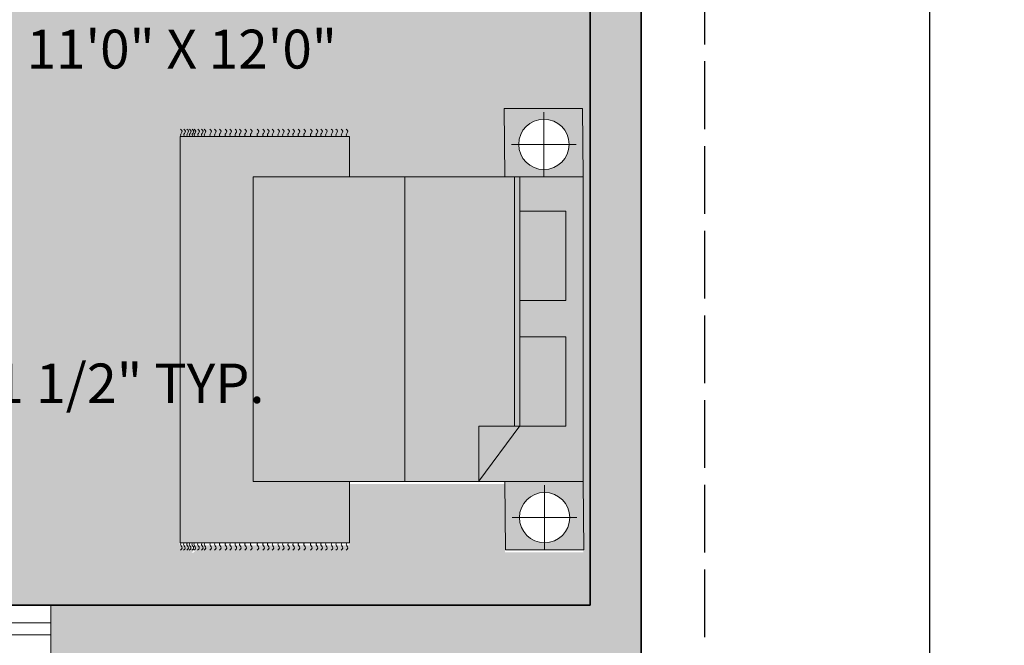
# Model space of a CAD drawing. Units: inches. Extents: x 1316 to 1777, y 813 to 1650.
# Tile 5 of 22: x 1603 to 1777, y 1126 to 1237. Entities that reach past the tile are written whole.
import ezdxf

# ---------------------------------------------------------------- set-up
doc = ezdxf.new("R2010")
doc.units = ezdxf.units.IN
doc.header["$MEASUREMENT"] = 0
doc.linetypes.add('ACAD_ISO02W100', pattern=[15, 12, -3])
for name, color, linetype, lineweight in [('A-ANNO-DIMS', 2, 'Continuous', 18), ('A-AREA-IDEN', 7, 'Continuous', 18), ('A-FURN-PATT', 23, 'Continuous', 13), ('A-WALL-PATT', 250, 'Continuous', 13), ('C-PROP', 8, 'ACAD_ISO02W100', 25), ('furniture', 23, 'Continuous', 18), ('walls', 250, 'Continuous', 35), ('windows', 141, 'Continuous', 18)]:
    doc.layers.add(name, color=color, linetype=linetype, lineweight=lineweight)
doc.layers.add('A-FLOR-PATT', color=254, linetype='Continuous', lineweight=13, true_color=0xfeeab9)
doc.styles.get("Standard").update_dxf_attribs({"font": 'arial.ttf'})
doc.dimstyles.get("Standard").update_dxf_attribs({"dimtxt": 7, "dimasz": 0.18, "dimexe": 0.18, "dimexo": 0.0625, "dimgap": 0.09, "dimtad": 0, "dimtih": 1, "dimtoh": 1, "dimzin": 0, "dimdsep": 46, "dimlunit": 3, "dimtxsty": 'Standard', "dimcen": 0.09, "dimadec": 0, "dimazin": 0, "dimtfac": 1, "dimtofl": 0, "dimtmove": 0, "dimatfit": 3, "dimfxl": 1, "dimtolj": 1, "dimtzin": 0, "dimarcsym": 0})

# ---------------------------------------------------------------- blocks, each defined once
blk = doc.blocks.new('CARPET')
at = {"layer": 'furniture'}
for p, q in [((-51.53, -98.11), (-51.53, -55.12)), ((-51.53, -55.12), (-41.27, -55.12)), ((36, -55.12), (51.55, -55.12)), ((51.55, -55.12), (51.55, -98.11)), ((51.55, -98.11), (-51.53, -98.11))]:
    blk.add_line(p, q, dxfattribs=at)
for points, knots in [([(-53.37, -55.99), (-53.22, -55.8), (-52.9, -55.41), (-52.34, -55.8), (-51.89, -56.08), (-51.65, -55.91), (-51.53, -55.83)], [0, 0, 0, 0, 0.653278, 1.290138, 1.740457, 2.114451, 2.114451, 2.114451, 2.114451]), ([(-53.37, -57.26), (-53.22, -57.07), (-52.9, -56.67), (-52.34, -57.07), (-51.89, -57.35), (-51.65, -57.17), (-51.53, -57.1)], [0, 0, 0, 0, 0.653278, 1.290138, 1.740457, 2.114451, 2.114451, 2.114451, 2.114451]), ([(53.37, -55.99), (53.22, -55.8), (52.9, -55.41), (52.34, -55.8), (51.89, -56.08), (51.65, -55.91), (51.53, -55.83)], [0, 0, 0, 0, 0.653278, 1.290138, 1.740457, 2.114451, 2.114451, 2.114451, 2.114451]), ([(53.37, -57.26), (53.22, -57.07), (52.9, -56.67), (52.34, -57.07), (51.89, -57.35), (51.65, -57.17), (51.53, -57.1)], [0, 0, 0, 0, 0.653278, 1.290138, 1.740457, 2.114451, 2.114451, 2.114451, 2.114451]), ([(-53.37, -58.59), (-53.22, -58.4), (-52.9, -58.01), (-52.34, -58.4), (-51.89, -58.68), (-51.65, -58.5), (-51.53, -58.43)], [0, 0, 0, 0, 0.653278, 1.290138, 1.740457, 2.114451, 2.114451, 2.114451, 2.114451]), ([(-53.37, -59.78), (-53.22, -59.58), (-52.9, -59.19), (-52.34, -59.58), (-51.89, -59.86), (-51.65, -59.69), (-51.53, -59.61)], [0, 0, 0, 0, 0.653278, 1.290138, 1.740457, 2.114451, 2.114451, 2.114451, 2.114451]), ([(53.37, -58.59), (53.22, -58.4), (52.9, -58.01), (52.34, -58.4), (51.89, -58.68), (51.65, -58.5), (51.53, -58.43)], [0, 0, 0, 0, 0.653278, 1.290138, 1.740457, 2.114451, 2.114451, 2.114451, 2.114451]), ([(53.37, -59.78), (53.22, -59.58), (52.9, -59.19), (52.34, -59.58), (51.89, -59.86), (51.65, -59.69), (51.53, -59.61)], [0, 0, 0, 0, 0.653278, 1.290138, 1.740457, 2.114451, 2.114451, 2.114451, 2.114451]), ([(-53.37, -61.22), (-53.22, -61.02), (-52.9, -60.63), (-52.34, -61.02), (-51.89, -61.3), (-51.65, -61.13), (-51.53, -61.05)], [0, 0, 0, 0, 0.653278, 1.290138, 1.740457, 2.114451, 2.114451, 2.114451, 2.114451]), ([(-53.37, -62.44), (-53.22, -62.25), (-52.9, -61.86), (-52.34, -62.25), (-51.89, -62.53), (-51.65, -62.36), (-51.53, -62.28)], [0, 0, 0, 0, 0.653278, 1.290138, 1.740457, 2.114451, 2.114451, 2.114451, 2.114451]), ([(53.37, -61.22), (53.22, -61.02), (52.9, -60.63), (52.34, -61.02), (51.89, -61.3), (51.65, -61.13), (51.53, -61.05)], [0, 0, 0, 0, 0.653278, 1.290138, 1.740457, 2.114451, 2.114451, 2.114451, 2.114451]), ([(53.37, -62.44), (53.22, -62.25), (52.9, -61.86), (52.34, -62.25), (51.89, -62.53), (51.65, -62.36), (51.53, -62.28)], [0, 0, 0, 0, 0.653278, 1.290138, 1.740457, 2.114451, 2.114451, 2.114451, 2.114451]), ([(-53.37, -63.63), (-53.22, -63.43), (-52.9, -63.04), (-52.34, -63.43), (-51.89, -63.72), (-51.65, -63.54), (-51.53, -63.46)], [0, 0, 0, 0, 0.653278, 1.290138, 1.740457, 2.114451, 2.114451, 2.114451, 2.114451]), ([(-53.37, -65.07), (-53.22, -64.87), (-52.9, -64.48), (-52.34, -64.87), (-51.89, -65.15), (-51.65, -64.98), (-51.53, -64.9)], [0, 0, 0, 0, 0.653278, 1.290138, 1.740457, 2.114451, 2.114451, 2.114451, 2.114451]), ([(53.37, -63.63), (53.22, -63.43), (52.9, -63.04), (52.34, -63.43), (51.89, -63.72), (51.65, -63.54), (51.53, -63.46)], [0, 0, 0, 0, 0.653278, 1.290138, 1.740457, 2.114451, 2.114451, 2.114451, 2.114451]), ([(53.37, -65.07), (53.22, -64.87), (52.9, -64.48), (52.34, -64.87), (51.89, -65.15), (51.65, -64.98), (51.53, -64.9)], [0, 0, 0, 0, 0.653278, 1.290138, 1.740457, 2.114451, 2.114451, 2.114451, 2.114451]), ([(-53.37, -66.76), (-53.22, -66.56), (-52.9, -66.17), (-52.34, -66.56), (-51.89, -66.84), (-51.65, -66.67), (-51.53, -66.59)], [0, 0, 0, 0, 0.653278, 1.290138, 1.740457, 2.114451, 2.114451, 2.114451, 2.114451]), ([(53.37, -66.76), (53.22, -66.56), (52.9, -66.17), (52.34, -66.56), (51.89, -66.84), (51.65, -66.67), (51.53, -66.59)], [0, 0, 0, 0, 0.653278, 1.290138, 1.740457, 2.114451, 2.114451, 2.114451, 2.114451]), ([(-53.37, -68.2), (-53.22, -68), (-52.9, -67.61), (-52.34, -68), (-51.89, -68.28), (-51.65, -68.11), (-51.53, -68.03)], [0, 0, 0, 0, 0.653278, 1.290138, 1.740457, 2.114451, 2.114451, 2.114451, 2.114451]), ([(-53.37, -69.53), (-53.22, -69.33), (-52.9, -68.94), (-52.34, -69.33), (-51.89, -69.61), (-51.65, -69.44), (-51.53, -69.36)], [0, 0, 0, 0, 0.653278, 1.290138, 1.740457, 2.114451, 2.114451, 2.114451, 2.114451]), ([(53.37, -68.2), (53.22, -68), (52.9, -67.61), (52.34, -68), (51.89, -68.28), (51.65, -68.11), (51.53, -68.03)], [0, 0, 0, 0, 0.653278, 1.290138, 1.740457, 2.114451, 2.114451, 2.114451, 2.114451]), ([(53.37, -69.53), (53.22, -69.33), (52.9, -68.94), (52.34, -69.33), (51.89, -69.61), (51.65, -69.44), (51.53, -69.36)], [0, 0, 0, 0, 0.653278, 1.290138, 1.740457, 2.114451, 2.114451, 2.114451, 2.114451]), ([(-53.37, -70.79), (-53.22, -70.6), (-52.9, -70.21), (-52.34, -70.6), (-51.89, -70.88), (-51.65, -70.7), (-51.53, -70.63)], [0, 0, 0, 0, 0.653278, 1.290138, 1.740457, 2.114451, 2.114451, 2.114451, 2.114451]), ([(-53.37, -72.12), (-53.22, -71.93), (-52.9, -71.54), (-52.34, -71.93), (-51.89, -72.21), (-51.65, -72.04), (-51.53, -71.96)], [0, 0, 0, 0, 0.653278, 1.290138, 1.740457, 2.114451, 2.114451, 2.114451, 2.114451]), ([(53.37, -70.79), (53.22, -70.6), (52.9, -70.21), (52.34, -70.6), (51.89, -70.88), (51.65, -70.7), (51.53, -70.63)], [0, 0, 0, 0, 0.653278, 1.290138, 1.740457, 2.114451, 2.114451, 2.114451, 2.114451]), ([(53.37, -72.12), (53.22, -71.93), (52.9, -71.54), (52.34, -71.93), (51.89, -72.21), (51.65, -72.04), (51.53, -71.96)], [0, 0, 0, 0, 0.653278, 1.290138, 1.740457, 2.114451, 2.114451, 2.114451, 2.114451]), ([(-53.37, -73.31), (-53.22, -73.11), (-52.9, -72.72), (-52.34, -73.11), (-51.89, -73.4), (-51.65, -73.22), (-51.53, -73.14)], [0, 0, 0, 0, 0.653278, 1.290138, 1.740457, 2.114451, 2.114451, 2.114451, 2.114451]), ([(-53.37, -74.75), (-53.22, -74.55), (-52.9, -74.16), (-52.34, -74.55), (-51.89, -74.83), (-51.65, -74.66), (-51.53, -74.58)], [0, 0, 0, 0, 0.653278, 1.290138, 1.740457, 2.114451, 2.114451, 2.114451, 2.114451]), ([(53.37, -73.31), (53.22, -73.11), (52.9, -72.72), (52.34, -73.11), (51.89, -73.4), (51.65, -73.22), (51.53, -73.14)], [0, 0, 0, 0, 0.653278, 1.290138, 1.740457, 2.114451, 2.114451, 2.114451, 2.114451]), ([(53.37, -74.75), (53.22, -74.55), (52.9, -74.16), (52.34, -74.55), (51.89, -74.83), (51.65, -74.66), (51.53, -74.58)], [0, 0, 0, 0, 0.653278, 1.290138, 1.740457, 2.114451, 2.114451, 2.114451, 2.114451]), ([(-53.37, -75.98), (-53.22, -75.78), (-52.9, -75.39), (-52.34, -75.78), (-51.89, -76.06), (-51.65, -75.89), (-51.53, -75.81)], [0, 0, 0, 0, 0.653278, 1.290138, 1.740457, 2.114451, 2.114451, 2.114451, 2.114451]), ([(-53.37, -77.16), (-53.22, -76.96), (-52.9, -76.57), (-52.34, -76.96), (-51.89, -77.25), (-51.65, -77.07), (-51.53, -76.99)], [0, 0, 0, 0, 0.653278, 1.290138, 1.740457, 2.114451, 2.114451, 2.114451, 2.114451]), ([(53.37, -75.98), (53.22, -75.78), (52.9, -75.39), (52.34, -75.78), (51.89, -76.06), (51.65, -75.89), (51.53, -75.81)], [0, 0, 0, 0, 0.653278, 1.290138, 1.740457, 2.114451, 2.114451, 2.114451, 2.114451]), ([(53.37, -77.16), (53.22, -76.96), (52.9, -76.57), (52.34, -76.96), (51.89, -77.25), (51.65, -77.07), (51.53, -76.99)], [0, 0, 0, 0, 0.653278, 1.290138, 1.740457, 2.114451, 2.114451, 2.114451, 2.114451]), ([(-53.37, -78.6), (-53.22, -78.4), (-52.9, -78.01), (-52.34, -78.4), (-51.89, -78.68), (-51.65, -78.51), (-51.53, -78.43)], [0, 0, 0, 0, 0.653278, 1.290138, 1.740457, 2.114451, 2.114451, 2.114451, 2.114451]), ([(-53.37, -80.29), (-53.22, -80.09), (-52.9, -79.7), (-52.34, -80.09), (-51.89, -80.37), (-51.65, -80.2), (-51.53, -80.12)], [0, 0, 0, 0, 0.653278, 1.290138, 1.740457, 2.114451, 2.114451, 2.114451, 2.114451]), ([(53.37, -78.6), (53.22, -78.4), (52.9, -78.01), (52.34, -78.4), (51.89, -78.68), (51.65, -78.51), (51.53, -78.43)], [0, 0, 0, 0, 0.653278, 1.290138, 1.740457, 2.114451, 2.114451, 2.114451, 2.114451]), ([(53.37, -80.29), (53.22, -80.09), (52.9, -79.7), (52.34, -80.09), (51.89, -80.37), (51.65, -80.2), (51.53, -80.12)], [0, 0, 0, 0, 0.653278, 1.290138, 1.740457, 2.114451, 2.114451, 2.114451, 2.114451]), ([(-53.37, -81.73), (-53.22, -81.53), (-52.9, -81.14), (-52.34, -81.53), (-51.89, -81.81), (-51.65, -81.64), (-51.53, -81.56)], [0, 0, 0, 0, 0.653278, 1.290138, 1.740457, 2.114451, 2.114451, 2.114451, 2.114451]), ([(53.37, -81.73), (53.22, -81.53), (52.9, -81.14), (52.34, -81.53), (51.89, -81.81), (51.65, -81.64), (51.53, -81.56)], [0, 0, 0, 0, 0.653278, 1.290138, 1.740457, 2.114451, 2.114451, 2.114451, 2.114451]), ([(-53.37, -83.06), (-53.22, -82.86), (-52.9, -82.47), (-52.34, -82.86), (-51.89, -83.14), (-51.65, -82.97), (-51.53, -82.89)], [0, 0, 0, 0, 0.653278, 1.290138, 1.740457, 2.114451, 2.114451, 2.114451, 2.114451]), ([(-53.37, -84.18), (-53.22, -83.99), (-52.9, -83.6), (-52.34, -83.99), (-51.89, -84.27), (-51.65, -84.09), (-51.53, -84.02)], [0, 0, 0, 0, 0.653278, 1.290138, 1.740457, 2.114451, 2.114451, 2.114451, 2.114451]), ([(53.37, -83.06), (53.22, -82.86), (52.9, -82.47), (52.34, -82.86), (51.89, -83.14), (51.65, -82.97), (51.53, -82.89)], [0, 0, 0, 0, 0.653278, 1.290138, 1.740457, 2.114451, 2.114451, 2.114451, 2.114451]), ([(53.37, -84.18), (53.22, -83.99), (52.9, -83.6), (52.34, -83.99), (51.89, -84.27), (51.65, -84.09), (51.53, -84.02)], [0, 0, 0, 0, 0.653278, 1.290138, 1.740457, 2.114451, 2.114451, 2.114451, 2.114451]), ([(-53.37, -85.51), (-53.22, -85.32), (-52.9, -84.93), (-52.34, -85.32), (-51.89, -85.6), (-51.65, -85.42), (-51.53, -85.35)], [0, 0, 0, 0, 0.653278, 1.290138, 1.740457, 2.114451, 2.114451, 2.114451, 2.114451]), ([(-53.37, -86.7), (-53.22, -86.5), (-52.9, -86.11), (-52.34, -86.5), (-51.89, -86.78), (-51.65, -86.61), (-51.53, -86.53)], [0, 0, 0, 0, 0.653278, 1.290138, 1.740457, 2.114451, 2.114451, 2.114451, 2.114451]), ([(53.37, -85.51), (53.22, -85.32), (52.9, -84.93), (52.34, -85.32), (51.89, -85.6), (51.65, -85.42), (51.53, -85.35)], [0, 0, 0, 0, 0.653278, 1.290138, 1.740457, 2.114451, 2.114451, 2.114451, 2.114451]), ([(53.37, -86.7), (53.22, -86.5), (52.9, -86.11), (52.34, -86.5), (51.89, -86.78), (51.65, -86.61), (51.53, -86.53)], [0, 0, 0, 0, 0.653278, 1.290138, 1.740457, 2.114451, 2.114451, 2.114451, 2.114451]), ([(-53.37, -88.14), (-53.22, -87.94), (-52.9, -87.55), (-52.34, -87.94), (-51.89, -88.22), (-51.65, -88.05), (-51.53, -87.97)], [0, 0, 0, 0, 0.653278, 1.290138, 1.740457, 2.114451, 2.114451, 2.114451, 2.114451]), ([(-53.37, -89.36), (-53.22, -89.17), (-52.9, -88.78), (-52.34, -89.17), (-51.89, -89.45), (-51.65, -89.28), (-51.53, -89.2)], [0, 0, 0, 0, 0.653278, 1.290138, 1.740457, 2.114451, 2.114451, 2.114451, 2.114451]), ([(53.37, -88.14), (53.22, -87.94), (52.9, -87.55), (52.34, -87.94), (51.89, -88.22), (51.65, -88.05), (51.53, -87.97)], [0, 0, 0, 0, 0.653278, 1.290138, 1.740457, 2.114451, 2.114451, 2.114451, 2.114451]), ([(53.37, -89.36), (53.22, -89.17), (52.9, -88.78), (52.34, -89.17), (51.89, -89.45), (51.65, -89.28), (51.53, -89.2)], [0, 0, 0, 0, 0.653278, 1.290138, 1.740457, 2.114451, 2.114451, 2.114451, 2.114451]), ([(-53.37, -90.55), (-53.22, -90.35), (-52.9, -89.96), (-52.34, -90.35), (-51.89, -90.64), (-51.65, -90.46), (-51.53, -90.38)], [0, 0, 0, 0, 0.653278, 1.290138, 1.740457, 2.114451, 2.114451, 2.114451, 2.114451]), ([(-53.37, -91.99), (-53.22, -91.79), (-52.9, -91.4), (-52.34, -91.79), (-51.89, -92.07), (-51.65, -91.9), (-51.53, -91.82)], [0, 0, 0, 0, 0.653278, 1.290138, 1.740457, 2.114451, 2.114451, 2.114451, 2.114451]), ([(-53.37, -92.69), (-53.22, -92.48), (-52.9, -92.08), (-52.35, -92.49), (-51.89, -92.77), (-51.65, -92.6), (-51.53, -92.52)], [0, 0, 0, 0, 0.663904, 1.307406, 1.757725, 2.131719, 2.131719, 2.131719, 2.131719]), ([(53.37, -90.55), (53.22, -90.35), (52.9, -89.96), (52.34, -90.35), (51.9, -90.63), (51.66, -90.47), (51.55, -90.4)], [0, 0, 0, 0, 0.653278, 1.290138, 1.740457, 2.0926, 2.0926, 2.0926, 2.0926]), ([(53.37, -91.99), (53.22, -91.79), (52.9, -91.4), (52.34, -91.79), (51.9, -92.07), (51.66, -91.91), (51.55, -91.83)], [0, 0, 0, 0, 0.653278, 1.290138, 1.740457, 2.0926, 2.0926, 2.0926, 2.0926]), ([(53.37, -92.69), (53.22, -92.49), (52.9, -92.09), (52.34, -92.49), (51.9, -92.77), (51.66, -92.61), (51.55, -92.53)], [0, 0, 0, 0, 0.656792, 1.295826, 1.746145, 2.098292, 2.098292, 2.098292, 2.098292]), ([(-53.37, -93.61), (-53.22, -93.42), (-52.9, -93.03), (-52.34, -93.42), (-51.89, -93.7), (-51.65, -93.52), (-51.53, -93.45)], [0, 0, 0, 0, 0.653278, 1.290138, 1.740457, 2.114451, 2.114451, 2.114451, 2.114451]), ([(-53.37, -94.55), (-53.22, -94.35), (-52.9, -93.96), (-52.34, -94.35), (-51.89, -94.63), (-51.65, -94.46), (-51.53, -94.38)], [0, 0, 0, 0, 0.653278, 1.290138, 1.740457, 2.114451, 2.114451, 2.114451, 2.114451]), ([(-53.37, -95.05), (-53.22, -94.85), (-52.9, -94.46), (-52.34, -94.85), (-51.89, -95.14), (-51.65, -94.96), (-51.53, -94.88)], [0, 0, 0, 0, 0.653278, 1.290138, 1.740457, 2.114451, 2.114451, 2.114451, 2.114451]), ([(53.37, -93.66), (53.22, -93.46), (52.9, -93.07), (52.34, -93.46), (51.9, -93.74), (51.66, -93.58), (51.55, -93.5)], [0, 0, 0, 0, 0.653278, 1.290138, 1.740457, 2.0926, 2.0926, 2.0926, 2.0926]), ([(53.37, -94.59), (53.22, -94.4), (52.9, -94.01), (52.34, -94.4), (51.9, -94.68), (51.66, -94.51), (51.55, -94.44)], [0, 0, 0, 0, 0.653278, 1.290138, 1.740457, 2.0926, 2.0926, 2.0926, 2.0926]), ([(53.37, -95.1), (53.22, -94.9), (52.9, -94.51), (52.34, -94.9), (51.9, -95.18), (51.66, -95.02), (51.55, -94.94)], [0, 0, 0, 0, 0.653278, 1.290138, 1.740457, 2.0926, 2.0926, 2.0926, 2.0926]), ([(-53.37, -95.73), (-53.22, -95.54), (-52.9, -95.15), (-52.34, -95.54), (-51.89, -95.82), (-51.65, -95.65), (-51.53, -95.57)], [0, 0, 0, 0, 0.653278, 1.290138, 1.740457, 2.114451, 2.114451, 2.114451, 2.114451]), ([(-53.37, -96.38), (-53.22, -96.18), (-52.9, -95.79), (-52.34, -96.18), (-51.89, -96.47), (-51.65, -96.29), (-51.53, -96.21)], [0, 0, 0, 0, 0.653278, 1.290138, 1.740457, 2.114451, 2.114451, 2.114451, 2.114451]), ([(-53.37, -97.17), (-53.22, -96.98), (-52.9, -96.59), (-52.34, -96.98), (-51.89, -97.26), (-51.65, -97.08), (-51.53, -97.01)], [0, 0, 0, 0, 0.653278, 1.290138, 1.740457, 2.114451, 2.114451, 2.114451, 2.114451]), ([(53.37, -95.78), (53.22, -95.58), (52.9, -95.19), (52.34, -95.58), (51.89, -95.86), (51.65, -95.69), (51.53, -95.61)], [0, 0, 0, 0, 0.653278, 1.290138, 1.740457, 2.114451, 2.114451, 2.114451, 2.114451]), ([(53.37, -96.43), (53.22, -96.23), (52.9, -95.84), (52.34, -96.23), (51.89, -96.51), (51.65, -96.34), (51.53, -96.26)], [0, 0, 0, 0, 0.653278, 1.290138, 1.740457, 2.114451, 2.114451, 2.114451, 2.114451]), ([(53.37, -97.22), (53.22, -97.02), (52.9, -96.63), (52.34, -97.02), (51.89, -97.3), (51.65, -97.13), (51.53, -97.05)], [0, 0, 0, 0, 0.653278, 1.290138, 1.740457, 2.114451, 2.114451, 2.114451, 2.114451]), ([(-53.37, -97.99), (-53.22, -97.79), (-52.9, -97.4), (-52.34, -97.79), (-51.89, -98.08), (-51.65, -97.9), (-51.53, -97.82)], [0, 0, 0, 0, 0.653278, 1.290138, 1.740457, 2.114451, 2.114451, 2.114451, 2.114451]), ([(53.37, -97.99), (53.22, -97.79), (52.9, -97.4), (52.34, -97.79), (51.89, -98.08), (51.65, -97.9), (51.53, -97.82)], [0, 0, 0, 0, 0.653278, 1.290138, 1.740457, 2.114451, 2.114451, 2.114451, 2.114451])]:
    blk.add_open_spline(points, degree=3, knots=knots, dxfattribs=at)
blk = doc.blocks.new('A$C58D270C6')
at = {"layer": 'furniture'}
for p, q in [((9.09, 124.13), (9.09, 108.87)), ((1.46, 116.5), (16.73, 116.5)), ((14.97, 94.84), (24.62, 107.92)), ((24.62, 94.93), (24.62, 107.92)), ((42.08, 108), (42.08, 36)), ((14.97, 94.93), (24.62, 94.93)), ((14.97, 94.84), (14.97, 36)), ((16.22, 94.93), (16.22, 36)), ((9.25, 36), (9.25, 20.74)), ((1.62, 28.37), (16.88, 28.37))]:
    blk.add_line(p, q, dxfattribs=at)
for points in [[(18.5, 108), (18.34, 124.13), (-0.16, 124.13), (0, 108)], [(0, 108), (77.91, 108), (77.91, 36), (0, 36)], [(4.09, 94.93), (14.97, 94.93), (14.97, 73.83), (4.09, 73.83)], [(4.09, 65.23), (14.97, 65.23), (14.97, 44.13), (4.09, 44.13)], [(18.65, 19.87), (18.5, 36), (0, 36), (0.16, 19.87)]]:
    blk.add_lwpolyline(points, close=True, dxfattribs=at)
for centre in [(9.09, 116.5), (9.25, 28.37)]:
    blk.add_circle(centre, 5.95, dxfattribs=at)
at = {"layer": 'furniture', "xscale": 0.9312884925094044, "yscale": 0.9312884925094044, "zscale": 0.9312884925094044, "rotation": 90}
blk.add_blockref('CARPET', (3.79, 74.47), dxfattribs=at)
blk = doc.blocks.new('*D32')
at = {"layer": 'A-ANNO-DIMS', "color": 0, "lineweight": -2, "transparency": 16777216}
for p, q in [((1508.99, 1175.95), (1508.99, 1171.97)), ((1534.72, 1175.95), (1534.72, 1171.97)), ((1509.17, 1172.15), (1534.54, 1172.15)), ((1534.72, 1172.15), (1534.9, 1172.15))]:
    blk.add_line(p, q, dxfattribs=at)
at = {"layer": 'A-ANNO-DIMS', "color": 0, "transparency": 16777216}
for points in [[(1509.17, 1172.18), (1509.17, 1172.12), (1508.99, 1172.15)], [(1534.54, 1172.18), (1534.54, 1172.12), (1534.72, 1172.15)]]:
    blk.add_solid(points, dxfattribs=at)
at = {"layer": 'Defpoints', "color": 0, "transparency": 16777216}
for p in [(1508.99, 1176.01), (1534.72, 1176.01), (1534.72, 1172.15)]:
    blk.add_point(p, dxfattribs=at)
at = {"layer": 'A-ANNO-DIMS', "color": 0, "transparency": 16777216, "insert": (1592.12, 1172.15), "char_height": 7, "attachment_point": 5}
blk.add_mtext('\\A1;ARMCHAIR 2\'-1 1/2" TYP.', dxfattribs=at)
blk = doc.blocks.new('*D51')
at = {"layer": 'A-ANNO-DIMS', "color": 0, "lineweight": -2, "transparency": 16777216}
for p, q in [((1713.24, 1575.37), (1764.48, 1575.37)), ((1764.3, 1575.19), (1764.3, 1306.92)), ((1764.3, 1031.35), (1764.3, 1299.62)), ((1713.24, 1031.17), (1764.48, 1031.17))]:
    blk.add_line(p, q, dxfattribs=at)
at = {"layer": 'A-ANNO-DIMS', "color": 0, "transparency": 16777216}
for points in [[(1764.27, 1575.19), (1764.33, 1575.19), (1764.3, 1575.37)], [(1764.27, 1031.35), (1764.33, 1031.35), (1764.3, 1031.17)]]:
    blk.add_solid(points, dxfattribs=at)
at = {"layer": 'Defpoints', "color": 0, "transparency": 16777216}
for p in [(1713.17, 1575.37), (1764.3, 1575.37), (1713.17, 1031.17)]:
    blk.add_point(p, dxfattribs=at)
at = {"layer": 'A-ANNO-DIMS', "color": 0, "transparency": 16777216, "insert": (1764.3, 1303.27), "char_height": 7, "attachment_point": 5}
blk.add_mtext('\\A1;45\'-4"', dxfattribs=at)

msp = doc.modelspace()

# ---------------------------------------------------------------- hatches: boundary and pattern name
at = {"layer": 'A-FLOR-PATT'}
h = msp.add_hatch(color=256, dxfattribs=at)
h.dxf.hatch_style = 1
h.paths.add_polyline_path([(1704.173, 1260.711), (1625.405, 1260.711), (1625.405, 1261.154), (1625.405, 1276.279), (1624.85, 1276.279), (1572.173, 1276.869), (1572.173, 1266.995), (1601.07, 1266.995), (1601.07, 1265.725), (1601.042, 1265.725, -0.4000145), (1572.173, 1237.955), (1572.173, 1132.869), (1704.173, 1132.869)])
edge = h.paths.add_edge_path(flags=0)
edge.add_spline(control_points=[(1634.063, 1215.447), (1634.008, 1215.524), (1633.887, 1215.694), (1634.084, 1216.011), (1634.356, 1216.402), (1634.084, 1216.621), (1633.946, 1216.732)], knot_values=[0, 0, 0, 0, 0.3739943, 0.8243137, 1.461173, 2.1144513, 2.1144513, 2.1144513, 2.1144513], degree=3, periodic=0)
edge.add_spline(control_points=[(1633.711, 1215.447), (1633.656, 1215.524), (1633.535, 1215.694), (1633.732, 1216.011), (1634.005, 1216.402), (1633.732, 1216.621), (1633.594, 1216.732)], knot_values=[0, 0, 0, 0, 0.3739943, 0.8243137, 1.461173, 2.1144513, 2.1144513, 2.1144513, 2.1144513], degree=3, periodic=0)
edge = h.paths.add_edge_path(flags=16)
edge.add_line((1631.459, 1215.447), (1661.482, 1215.447))
edge.add_line((1661.482, 1215.447), (1661.482, 1208.307))
edge.add_line((1661.482, 1208.307), (1688.953, 1208.307))
edge.add_line((1688.953, 1208.307), (1688.837, 1220.405))
edge.add_line((1688.837, 1220.405), (1702.711, 1220.405))
edge.add_line((1702.711, 1220.405), (1702.827, 1208.307))
edge.add_line((1702.827, 1208.307), (1702.827, 1154.307))
edge.add_line((1702.827, 1154.307), (1702.944, 1142.208))
edge.add_line((1702.944, 1142.208), (1689.07, 1142.208))
edge.add_line((1689.07, 1142.208), (1688.953, 1154.307))
edge.add_line((1688.953, 1154.307), (1661.482, 1154.307))
edge.add_line((1661.482, 1154.307), (1661.482, 1143.444))
edge.add_line((1661.482, 1143.444), (1634.022, 1143.444))
edge.add_spline(control_points=[(1634.022, 1143.444), (1633.972, 1143.371), (1633.857, 1143.204), (1634.053, 1142.892), (1634.324, 1142.501), (1634.052, 1142.282), (1633.914, 1142.172)], knot_values=[0, 0, 0, 0, 0.3521435, 0.8024629, 1.4393222, 2.0926005, 2.0926005, 2.0926005, 2.0926005], degree=3, periodic=0)
edge.add_spline(control_points=[(1633.562, 1142.172), (1633.7, 1142.282), (1633.973, 1142.501), (1633.701, 1142.892), (1633.505, 1143.204), (1633.62, 1143.371), (1633.67, 1143.444)], knot_values=[0, 0, 0, 0, 0.6532783, 1.2901376, 1.740457, 2.0926005, 2.0926005, 2.0926005, 2.0926005], degree=3, periodic=0)
edge.add_line((1633.67, 1143.444), (1631.459, 1143.444))
edge.add_line((1631.459, 1143.444), (1631.459, 1215.447))
h.paths.add_polyline_path([(1691.549, 1164.108), (1691.597, 1164.173), (1691.597, 1202.209), (1699.757, 1202.209), (1699.757, 1186.386), (1691.597, 1186.386), (1691.597, 1179.931), (1699.757, 1179.931), (1699.757, 1164.108), (1691.549, 1164.108), (1684.365, 1154.365), (1684.365, 1164.108)], flags=0)
h.paths.add_polyline_path([(1691.424, 1214.03, -1), (1700.356, 1214.03, -1)], flags=0)
h.paths.add_polyline_path([(1691.541, 1147.932, -1), (1700.473, 1147.932, -1)], flags=0)
h.paths.add_polyline_path([(1601.042, 1265.725), (1572.029, 1265.725), (1572.029, 1266.995), (1567.673, 1266.995), (1567.673, 1237.955), (1572.029, 1237.955, 0.4014527)])
at = {"layer": 'A-FURN-PATT'}
h = msp.add_hatch(color=256, dxfattribs=at)
h.dxf.hatch_style = 1
h.paths.add_polyline_path([(1689.016, 1154.742), (1702.89, 1154.742), (1703.007, 1142.644), (1696.069, 1142.644), (1696.069, 1143.901, 0.4142136), (1700.536, 1148.367, 1), (1691.603, 1148.367, 0.4142136), (1696.069, 1143.901), (1696.069, 1142.644), (1689.132, 1142.644)])
h.paths.add_polyline_path([(1691.611, 1164.543), (1699.819, 1164.543), (1699.819, 1180.366), (1691.659, 1180.366), (1691.659, 1186.822), (1699.819, 1186.822), (1699.819, 1202.644), (1691.659, 1202.644), (1691.659, 1208.742), (1702.89, 1208.742), (1702.89, 1154.742), (1684.427, 1154.742), (1684.427, 1154.8)])
h.paths.add_polyline_path([(1691.487, 1214.465, 0.4142136), (1695.953, 1209.999), (1695.953, 1208.742), (1689.016, 1208.742), (1688.899, 1220.84), (1702.773, 1220.84), (1702.89, 1208.742), (1695.953, 1208.742), (1695.953, 1209.999, 0.4142136), (1700.419, 1214.465, 1)])
h = msp.add_hatch(color=256, dxfattribs=at)
h.dxf.hatch_style = 1
h.paths.add_polyline_path([(1691.659, 1180.366), (1699.819, 1180.366), (1699.819, 1164.543), (1691.659, 1164.543)])
h.paths.add_polyline_path([(1691.659, 1202.644), (1699.819, 1202.644), (1699.819, 1186.822), (1691.659, 1186.822)])
h.paths.add_polyline_path([(1631.521, 1215.882), (1661.545, 1215.882), (1661.545, 1208.742), (1644.461, 1208.742), (1644.461, 1154.742), (1661.545, 1154.742), (1661.545, 1143.879), (1631.521, 1143.879)])
h = msp.add_hatch(color=256, dxfattribs=at)
h.dxf.hatch_style = 1
h.paths.add_polyline_path([(1644.461, 1208.742), (1671.331, 1208.742), (1671.331, 1154.742), (1644.461, 1154.742)])
h.paths.add_polyline_path([(1671.331, 1208.742), (1690.727, 1208.742), (1690.727, 1164.543), (1684.427, 1164.543), (1684.427, 1154.742), (1671.331, 1154.742)])
h = msp.add_hatch(color=256, dxfattribs=at)
h.dxf.hatch_style = 1
h.paths.add_polyline_path([(1684.427, 1164.543), (1691.611, 1164.543), (1684.427, 1154.8)])
h.paths.add_polyline_path([(1690.727, 1208.742), (1691.659, 1208.742), (1691.659, 1164.609), (1691.611, 1164.543), (1690.727, 1164.543)])
h = msp.add_hatch(color=256, dxfattribs=at)
h.dxf.hatch_style = 1
h.paths.add_polyline_path([(1684.402, 1164.251), (1691.585, 1164.251), (1684.402, 1154.508)])
h.paths.add_polyline_path([(1690.702, 1208.45), (1691.634, 1208.45), (1691.634, 1164.317), (1691.585, 1164.251), (1690.702, 1164.251)])
at = {"layer": 'A-WALL-PATT'}
h = msp.add_hatch(color=256, dxfattribs=at)
h.dxf.hatch_style = 1
h.paths.add_polyline_path([(1713.173, 1281.369), (1656.173, 1281.369), (1656.173, 1298.258), (1651.673, 1298.258), (1651.673, 1281.369), (1567.673, 1281.369), (1567.673, 1266.995), (1572.173, 1266.995), (1572.173, 1276.869), (1704.173, 1276.869), (1704.173, 1132.869), (1608.64, 1132.869), (1608.64, 1123.869), (1704.173, 1123.869), (1704.173, 1040.173), (1652.869, 1040.173), (1652.869, 1031.173), (1713.173, 1031.173), (1713.173, 1040.173)])
h.paths.add_polyline_path([(1572.173, 1237.955), (1567.673, 1237.955), (1567.673, 1123.869), (1583.146, 1123.869), (1583.146, 1132.869), (1572.173, 1132.869)], flags=17)
h.paths.add_polyline_path([(1510.345, 1566.369), (1524.171, 1566.369), (1524.171, 1571.985), (1524.171, 1575.369), (1445.955, 1575.369), (1445.955, 1566.369), (1505.845, 1566.369), (1505.845, 1469.591), (1510.345, 1469.591), (1510.345, 1471.869), (1529.081, 1471.869), (1529.081, 1476.369), (1510.345, 1476.369)])
h.paths.add_polyline_path([(1609.722, 1575.369), (1545.119, 1575.369), (1545.119, 1566.369), (1570.345, 1566.369), (1570.345, 1476.369), (1562.477, 1476.369), (1562.477, 1471.869), (1570.345, 1471.869), (1570.345, 1469.591), (1574.845, 1469.591), (1574.845, 1566.369), (1609.722, 1566.369)])
h.paths.add_polyline_path([(1713.173, 1575.369), (1655.233, 1575.369), (1655.233, 1566.369), (1704.173, 1566.369), (1704.173, 1434.369), (1574.845, 1434.369), (1574.845, 1440.551), (1574.701, 1440.551), (1570.345, 1440.551), (1570.345, 1429.869), (1597.673, 1429.869), (1597.673, 1408.281), (1602.173, 1408.281), (1602.173, 1429.869), (1704.173, 1429.869), (1704.173, 1410.704), (1707.375, 1410.704), (1713.173, 1410.704)])
h.paths.add_polyline_path([(1713.173, 1383.676), (1704.173, 1383.676), (1704.173, 1369.869), (1602.173, 1369.869), (1602.173, 1379.241), (1597.673, 1379.241), (1597.673, 1365.369), (1713.173, 1365.369)])
h.paths.add_polyline_path([(1444.564, 1429.869), (1510.345, 1429.869), (1510.345, 1440.551), (1505.845, 1440.551), (1505.845, 1434.369), (1386.064, 1434.369), (1386.064, 1566.369), (1400.445, 1566.369), (1400.445, 1575.369), (1377.064, 1575.369), (1377.064, 1412.813), (1380.509, 1412.813), (1386.064, 1412.813), (1386.064, 1429.869), (1440.064, 1429.869), (1440.064, 1401.229), (1444.564, 1401.229)])
h.paths.add_polyline_path([(1444.564, 1372.189), (1440.064, 1372.189), (1440.064, 1369.869), (1386.064, 1369.869), (1386.064, 1378.758), (1377.064, 1378.758), (1377.064, 1349.201), (1381.118, 1349.201), (1386.064, 1349.201), (1386.064, 1365.369), (1440.064, 1365.369), (1440.064, 1322.882), (1444.564, 1322.882)])
h.paths.add_polyline_path([(1510.564, 1295.094), (1506.064, 1295.094), (1506.064, 1245.369), (1386.064, 1245.369), (1386.064, 1272.582), (1377.064, 1272.582), (1377.064, 1212.905), (1380.1, 1212.905), (1386.064, 1212.905), (1386.064, 1240.869), (1510.564, 1240.869)])
h.paths.add_polyline_path([(1386.064, 1163.761), (1377.064, 1163.761), (1377.064, 1063.869), (1419.363, 1063.869), (1419.363, 1072.869), (1386.064, 1072.869)])
h.paths.add_polyline_path([(1510.564, 1072.869), (1469.381, 1072.869), (1469.381, 1063.869), (1501.564, 1063.869), (1501.564, 1033.023), (1501.564, 1031.173), (1540.829, 1031.173), (1540.829, 1036.182, -0.0299535), (1541.068, 1040.173), (1510.564, 1040.173)])
h.paths.add_polyline_path([(1607.369, 1040.173), (1574.225, 1040.173), (1574.225, 1036.182), (1574.225, 1031.173), (1607.369, 1031.173)], flags=17)
h.paths.add_polyline_path([(1637.054, 1040.173), (1624.706, 1040.173), (1624.706, 1031.173), (1637.054, 1031.173)], flags=17)

# ---------------------------------------------------------------- linework, layer by layer
at = {"layer": 'C-PROP'}
msp.add_line((1724.399, 1604.173), (1724.399, 1040.173), dxfattribs=at)
at = {"layer": 'walls'}
for p, q in [((1713.173, 1575.369), (1713.173, 1040.173)), ((1704.173, 1276.869), (1704.173, 1132.869)), ((1572.173, 1132.869), (1704.173, 1132.869))]:
    msp.add_line(p, q, dxfattribs=at)
at = {"layer": 'windows'}
for p, q in [((1608.64, 1132.869), (1583.146, 1132.869)), ((1608.64, 1123.869), (1608.64, 1132.869)), ((1583.146, 1129.718), (1608.64, 1129.718)), ((1608.64, 1129.718), (1608.64, 1127.621)), ((1608.64, 1127.621), (1583.146, 1127.621))]:
    msp.add_line(p, q, dxfattribs=at)

# ---------------------------------------------------------------- block references
at = {"layer": 'furniture', "xscale": 0.7500000390647866, "yscale": 0.7500000390647866, "zscale": 0.7500000390647866, "rotation": 180}
msp.add_blockref('A$C58D270C6', (1702.89, 1235.742), dxfattribs=at)

# ---------------------------------------------------------------- texts
at = {"layer": 'A-AREA-IDEN'}
msp.add_text('11\'0" X 12\'0"', height=6.88202, dxfattribs=at).set_placement((1604.33, 1227.895))

# ---------------------------------------------------------------- dimensions: what is measured, and where the dimension line sits
at = {"layer": 'A-ANNO-DIMS'}
dim = msp.add_linear_dim(base=(1764.299, 1575.369), p1=(1713.173, 1031.173), p2=(1713.173, 1575.369), angle=90, dimstyle='Standard', override={"dimdec": 1, "dimlfac": 1, "dimrnd": 0, "dimzin": 1, "dimdsep": 46, "dimlunit": 4, "dimfrac": 2}, dxfattribs=at)
dim.commit()
dim.dimension.update_dxf_attribs({"geometry": '*D51', "text_midpoint": (1764.299, 1303.271)})
dim = msp.add_linear_dim(base=(1534.725, 1172.148), p1=(1508.987, 1176.008), p2=(1534.725, 1176.008), text='ARMCHAIR <> TYP.', dimstyle='Standard', override={"dimdec": 1, "dimlfac": 1, "dimrnd": 0, "dimzin": 1, "dimdsep": 46, "dimlunit": 4, "dimfrac": 2}, dxfattribs=at)
dim.commit()
dim.dimension.update_dxf_attribs({"geometry": '*D32', "text_midpoint": (1592.124, 1172.148)})

doc.saveas('drawing.dxf')
